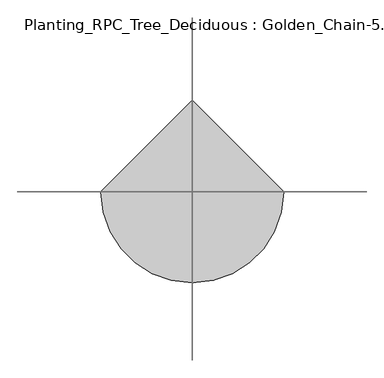
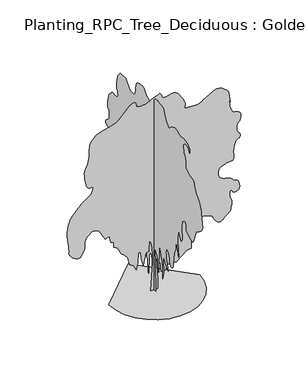
"""IFC4 building model written with IfcOpenShell, lengths in millimetres: geographic element geometry, Planting_RPC_Tree_Deciduous : Golden_Chain-5.5_Meters."""

from ifc_helpers import new_model, si_unit, origin, place, context, project, spatial, triangles, source, transform, mapped, element, save


def planting_rpc_tree_deciduous_golden_chain_5_5_meters_a00e3d8d(model_context):
    return source(origin(), model_context, "Body", "Tessellation", [
        triangles([(-0.0021492, 84.2526244, 0.0017055), (-0.0021492, -79.7118133, 0.0017055), (-0.0021492, -55.1171344, 770.634066), (-0.0021492, -30.52271, 1205.1392303), (-0.0021492, -128.9011709, 1090.3649134), (-0.0021492, -161.6941638, 983.7871164), (-0.0021492, -161.6941638, 778.8331295), (-0.0021492, -202.6851937, 614.866975), (-0.0021492, -227.2798771, 1410.0957607), (-0.0021492, -292.8648455, 1254.3285244), (-0.0021492, -391.2435608, 934.5977497), (-0.0021492, -407.6416878, 557.4810519), (-0.0021492, -448.631991, 754.2384825), (-0.0021492, -424.0373076, 1123.1586239), (-0.0021492, -399.4426243, 1229.73395), (-0.0021492, -563.406308, 1024.7799631), (-0.0021492, -645.3893852, 910.0031027), (-0.0021492, -571.6053715, 1164.1489271), (-0.0021492, -566.3701896, 1202.7023878), (-0.0021492, -561.3514189, 1240.6803749), (-0.0021492, -556.7629998, 1277.5125744), (-0.0021492, -552.8188002, 1312.6235126), (-0.0021492, -549.7352311, 1345.4427303), (-0.0021492, -547.7261968, 1375.3897396), (-0.0021492, -547.0106881, 1401.8966972), (-0.0021492, -548.2049103, 1425.0577835), (-0.0021492, -551.5507453, 1445.6369053), (-0.0021492, -556.6891671, 1464.0644142), (-0.0021492, -563.2636931, 1480.7706619), (-0.0021492, -570.9127902, 1496.1886162), (-0.0021492, -579.2773596, 1510.7457218), (-0.0021492, -588.000955, 1524.870005), (-0.0021492, -615.9185823, 1493.2475166), (-0.0021492, -642.6878059, 1461.6276443), (-0.0021492, -667.1627655, 1430.0051559), (-0.0021492, -688.1977461, 1398.3828129), (-0.0021492, -704.6417278, 1366.7627953), (-0.0021492, -715.3489231, 1335.1404522), (-0.0021492, -719.1734716, 1303.5179638), (-0.0021492, -720.8463346, 1273.0922047), (-0.0021492, -725.5315138, 1244.8155876), (-0.0021492, -732.7248247, 1218.3341372), (-0.0021492, -741.92717, 1193.2836313), (-0.0021492, -752.6342926, 1169.3103127), (-0.0021492, -764.3473131, 1146.0549734), (-0.0021492, -776.5592857, 1123.1586239), (-0.0021492, -799.2416948, 1123.4208899), (-0.0021492, -820.9921841, 1125.2619112), (-0.0021492, -840.8787609, 1130.2577545), (-0.0021492, -857.9695055, 1139.9845591), (-0.0021492, -871.3299545, 1156.0211529), (-0.0021492, -880.0306589, 1179.9486895), (-0.0021492, -883.1370827, 1213.3382938), (-0.0021492, -884.8100183, 1255.5711811), (-0.0021492, -889.4951975, 1304.2589069), (-0.0021492, -896.6885084, 1358.3243568), (-0.0021492, -905.890781, 1416.6931778), (-0.0021492, -916.5979763, 1478.2854939), (-0.0021492, -928.3109241, 1542.0320389), (-0.0021492, -940.5255129, 1606.8530823), (-0.0021492, -1006.1104631, 1762.6177025), (-0.0021492, -1030.7051828, 2041.3582466), (-0.0021492, -1137.2829798, 1615.049675), (-0.0021492, -1096.2901331, 2033.1591831), (-0.0021492, -1120.8847801, 2385.683741), (-0.0021492, -1260.2563602, 2139.7369801), (-0.0021492, -1270.7241806, 2153.8612633), (-0.0021492, -1280.7616493, 2168.4185143), (-0.0021492, -1289.9410309, 2183.833707), (-0.0021492, -1297.8295029, 2200.5425709), (-0.0021492, -1303.9940975, 2218.9700798), (-0.0021492, -1308.0095501, 2239.5492016), (-0.0021492, -1309.4456543, 2262.7104332), (-0.0021492, -1307.6275967, 2290.0779488), (-0.0021492, -1302.9424175, 2322.0339924), (-0.0021492, -1296.5385933, 2357.1449306), (-0.0021492, -1289.5590775, 2393.9769848), (-0.0021492, -1283.1526371, 2431.0969574), (-0.0021492, -1278.467458, 2467.0685989), (-0.0021492, -1276.6520164, 2500.4581306), (-0.0021492, -1277.8461296, 2532.7959824), (-0.0021492, -1281.1946171, 2566.4378242), (-0.0021492, -1286.3329662, 2601.1438454), (-0.0021492, -1292.9049488, 2636.6899315), (-0.0021492, -1300.5540459, 2672.8984772), (-0.0021492, -1308.9186516, 2709.5395546), (-0.0021492, -1317.642247, 2746.4099785), (-0.0021492, -1349.0965771, 2763.5973015), (-0.0021492, -1379.5477707, 2778.4931946), (-0.0021492, -1407.98993, 2788.7803574), (-0.0021492, -1433.4223892, 2792.1923584), (-0.0021492, -1454.8366344, 2786.4377678), (-0.0021492, -1471.2349068, 2769.1992851), (-0.0021492, -1481.6059307, 2738.2107697), (-0.0021492, -1484.4043064, 2701.9007767), (-0.0021492, -1481.8937038, 2669.6135033), (-0.0021492, -1478.8100258, 2640.331279), (-0.0021492, -1479.8871403, 2613.0602692), (-0.0021492, -1489.8533924, 2586.7825127), (-0.0021492, -1513.4448303, 2560.530336), (-0.0021492, -1555.3924152, 2533.2517685), (-0.0021492, -1606.8990097, 2505.0720932), (-0.0021492, -1655.2531803, 2478.4681938), (-0.0021492, -1699.3015091, 2456.025087), (-0.0021492, -1737.903368, 2440.3222664), (-0.0021492, -1769.9078098, 2433.9411152), (-0.0021492, -1794.1663582, 2439.4615631), (-0.0021492, -1809.5357689, 2459.4679001), (-0.0021492, -1957.1037964, 2820.1761154), (-0.0021492, -2096.4729057, 2918.565168), (-0.0021492, -2133.9034698, 2947.2108032), (-0.0021492, -2168.0339447, 2976.9770096), (-0.0021492, -2197.5760368, 3008.067263), (-0.0021492, -2221.2388367, 3040.5580124), (-0.0021492, -2237.731144, 3074.6530243), (-0.0021492, -2245.7621944, 3110.4540367), (-0.0021492, -2244.0409332, 3148.1136566), (-0.0021492, -2235.2459759, 3194.9401588), (-0.0021492, -2223.8691994, 3254.6760475), (-0.0021492, -2211.3439465, 3322.1530334), (-0.0021492, -2199.1064667, 3392.2016647), (-0.0021492, -2188.5902481, 3459.6786507), (-0.0021492, -2181.2289242, 3519.4145393), (-0.0021492, -2178.455983, 3566.2154617), (-0.0021492, -2170.3281361, 3608.6878693), (-0.0021492, -2147.5744377, 3658.060437), (-0.0021492, -2112.6316578, 3713.1367264), (-0.0021492, -2067.93395, 3772.8220367), (-0.0021492, -2015.9257874, 3835.9446373), (-0.0021492, -1959.038998, 3901.3845383), (-0.0021492, -1899.7154388, 3967.9447197), (-0.0021492, -1842.3295521, 4197.493499), (-0.0021492, -1629.1739582, 4246.6878799), (-0.0021492, -1457.0138271, 4328.6532257), (-0.0021492, -1458.3505188, 4335.1970123), (-0.0021492, -1461.6963902, 4352.7409996), (-0.0021492, -1466.0480141, 4378.3568779), (-0.0021492, -1470.3971672, 4408.9634399), (-0.0021492, -1473.7428932, 4441.6067963), (-0.0021492, -1475.0823463, 4473.206321), (-0.0021492, -1473.409338, 4500.8337044), (-0.0021492, -1467.7438408, 4526.8568253), (-0.0021492, -1458.2079403, 4555.4518822), (-0.0021492, -1445.4434578, 4586.2110512), (-0.0021492, -1430.0994816, 4618.7018005), (-0.0021492, -1412.8176876, 4652.465728), (-0.0021492, -1394.2476002, 4687.1208801), (-0.0021492, -1375.0306046, 4722.1832748), (-0.0021492, -1342.2369667, 4918.9358002), (-0.0021492, -1448.8147636, 5009.1256439), (-0.0021492, -1579.9871349, 4984.5283081), (-0.0021492, -1653.7686779, 4877.9400467), (-0.0021492, -1653.7686779, 4976.32939), (-0.0021492, -1538.9942883, 5082.8914902), (-0.0021492, -1350.4360302, 5107.488826), (-0.0021492, -1202.86793, 5074.692572), (-0.0021492, -1055.2998299, 5156.6834976), (-0.0021492, -948.7220329, 5164.8824158), (-0.0021492, -940.8820318, 5161.1390396), (-0.0021492, -920.1373678, 5151.1070938), (-0.0021492, -890.6410578, 5136.4911255), (-0.0021492, -856.5588358, 5118.9980072), (-0.0021492, -822.0437914, 5100.3340302), (-0.0021492, -791.2591152, 5082.280481), (-0.0021492, -768.3627657, 5066.4936539), (-0.0021492, -752.5401123, 5050.8591431), (-0.0021492, -739.1542288, 5033.7991379), (-0.0021492, -726.6289759, 5017.8844116), (-0.0021492, -713.388287, 5005.688063), (-0.0021492, -697.8532614, 4999.805864), (-0.0021492, -678.4454344, 5002.8359116), (-0.0021492, -653.5859053, 5017.2989822), (-0.0021492, -627.152853, 5039.5790176), (-0.0021492, -603.7294644, 5064.0234558), (-0.0021492, -582.8141713, 5090.2247635), (-0.0021492, -563.9079125, 5117.8777267), (-0.0021492, -546.5090836, 5146.6253906), (-0.0021492, -530.1109202, 5176.0608032), (-0.0021492, -514.2169413, 5205.8775879), (-0.0021492, -415.8382442, 5410.8290314), (-0.0021492, -169.8924643, 5451.8247849), (-0.0021492, -163.845268, 5451.6718872), (-0.0021492, -147.6161895, 5450.6789246), (-0.0021492, -124.0728773, 5447.9540909), (-0.0021492, -96.0842423, 5442.6323227), (-0.0021492, -66.5181782, 5433.8985535), (-0.0021492, -38.242574, 5420.8359787), (-0.0021492, -14.1260636, 5402.6301132), (-0.0021492, 3.3458591, 5384.2457703), (-0.0021492, 15.2248417, 5370.0373352), (-0.0021492, 23.9488607, 5358.0956223), (-0.0021492, 31.9557666, 5346.6114395), (-0.0021492, 41.6836385, 5333.6761826), (-0.0021492, 55.5706315, 5317.4312439), (-0.0021492, 76.0543103, 5296.0418518), (-0.0021492, 97.1353591, 5271.2921997), (-0.0021492, 113.1971422, 5247.5349289), (-0.0021492, 127.251426, 5226.7827072), (-0.0021492, 142.3092006, 5211.0464584), (-0.0021492, 161.3827366, 5202.3638489), (-0.0021492, 187.4830512, 5202.6946426), (-0.0021492, 223.6221243, 5214.0770874), (-0.0021492, 264.3514152, 5233.7851868), (-0.0021492, 302.4974698, 5257.3895599), (-0.0021492, 338.4919115, 5284.2018768), (-0.0021492, 372.7676173, 5313.5861298), (-0.0021492, 405.7523409, 5344.9307281), (-0.0021492, 437.8764338, 5377.549086), (-0.0021492, 469.5676317, 5410.8290314), (-0.0021492, 492.4664884, 5419.4866425), (-0.0021492, 515.7217913, 5427.329187), (-0.0021492, 539.6951826, 5433.618338), (-0.0021492, 564.7456521, 5437.5396103), (-0.0021492, 591.2271389, 5438.3035172), (-0.0021492, 619.503756, 5435.1205719), (-0.0021492, 649.9294424, 5427.227449), (-0.0021492, 681.4067362, 5417.9076691), (-0.0021492, 712.0260155, 5409.8616486), (-0.0021492, 740.9213448, 5401.4080948), (-0.0021492, 767.2373257, 5390.7895569), (-0.0021492, 790.1107115, 5376.3014877), (-0.0021492, 808.683415, 5356.2364334), (-0.0021492, 822.0921896, 5328.8381058), (-0.0021492, 831.6764883, 5297.4679276), (-0.0021492, 839.5394531, 5266.5052826), (-0.0021492, 845.9687845, 5235.9240097), (-0.0021492, 851.252401, 5205.5973724), (-0.0021492, 855.6727707, 5175.5259521), (-0.0021492, 859.5227537, 5145.5556885), (-0.0021492, 863.0824928, 5115.6877441), (-0.0021492, 868.5086151, 5085.9982773), (-0.0021492, 874.8667299, 5057.4029297), (-0.0021492, 883.0887571, 5030.9469864), (-0.0021492, 894.1065439, 5007.6995682), (-0.0021492, 908.8546989, 4988.7803741), (-0.0021492, 928.2625986, 4975.2085281), (-0.0021492, 953.2646336, 4968.1298904), (-0.0021492, 983.5707052, 4964.7946289), (-0.0021492, 1017.0341423, 4962.6302261), (-0.0021492, 1051.7859455, 4962.7319641), (-0.0021492, 1085.9648912, 4966.2968628), (-0.0021492, 1117.7070671, 4974.4446213), (-0.0021492, 1145.1459446, 4988.3478424), (-0.0021492, 1166.417684, 5009.1256439), (-0.0021492, 1187.9516893, 5037.6186722), (-0.0021492, 1215.2250973, 5071.5857849), (-0.0021492, 1244.9327316, 5107.4126678), (-0.0021492, 1273.7822788, 5141.5326782), (-0.0021492, 1298.4736496, 5170.3315018), (-0.0021492, 1315.7070454, 5190.2436584), (-0.0021492, 1322.1822315, 5197.6786697), (-0.0021492, 1576.3282013, 5181.2802521), (-0.0021492, 1674.7067894, 5058.2941544), (-0.0021492, 1679.9878624, 5049.3057495), (-0.0021492, 1685.3427681, 5039.1209061), (-0.0021492, 1690.8402523, 5026.4658646), (-0.0021492, 1696.5540024, 5010.1691849), (-0.0021492, 1702.550584, 4988.9844315), (-0.0021492, 1708.9087715, 4961.7134216), (-0.0021492, 1715.6971653, 4927.1347183), (-0.0021492, 1722.2461842, 4888.9655365), (-0.0021492, 1727.9346451, 4851.6622902), (-0.0021492, 1732.9075974, 4815.0467926), (-0.0021492, 1737.3050034, 4779.0420135), (-0.0021492, 1741.2720577, 4743.4447678), (-0.0021492, 1744.9541004, 4708.1530266), (-0.0021492, 1748.4909485, 4672.9888939), (-0.0021492, 1731.0895397, 4648.3406891), (-0.0021492, 1714.6938835, 4623.4122688), (-0.0021492, 1700.3047909, 4597.923999), (-0.0021492, 1688.927869, 4571.5442139), (-0.0021492, 1681.5665451, 4544.0444389), (-0.0021492, 1679.2239555, 4515.0930084), (-0.0021492, 1682.9058529, 4484.4355774), (-0.0021492, 1691.9172215, 4457.546521), (-0.0021492, 1704.7989933, 4438.9587021), (-0.0021492, 1721.4110607, 4426.9911186), (-0.0021492, 1741.6082291, 4419.8869011), (-0.0021492, 1765.2454491, 4415.940049), (-0.0021492, 1792.1827583, 4413.4448524), (-0.0021492, 1822.2749622, 4410.6438606), (-0.0021492, 1851.5776794, 4410.5165428), (-0.0021492, 1877.0101387, 4414.7180305), (-0.0021492, 1899.7154388, 4419.4540787), (-0.0021492, 1920.8445271, 4421.0583412), (-0.0021492, 1941.543409, 4415.787442), (-0.0021492, 1962.9577995, 4399.8985863), (-0.0021492, 1986.2386459, 4369.6483978), (-0.0021492, 2009.8529022, 4339.0165466), (-0.0021492, 2031.6034641, 4320.2758301), (-0.0021492, 2051.6326195, 4307.2641243), (-0.0021492, 2070.0855629, 4293.8451759), (-0.0021492, 2087.1025475, 4273.8059921), (-0.0021492, 2102.8309479, 4241.0097382), (-0.0021492, 2117.4110172, 4189.2942902), (-0.0021492, 2130.4608021, 4132.1300468), (-0.0021492, 2141.5041687, 4085.4564423), (-0.0021492, 2150.5383556, 4046.6762512), (-0.0021492, 2157.5661243, 4013.1925392), (-0.0021492, 2162.5848587, 3982.4330795), (-0.0021492, 2165.5945587, 3951.8012283), (-0.0021492, 2166.6004566, 3918.7503387), (-0.0021492, 2163.9700939, 3888.1437767), (-0.0021492, 2156.60877, 3865.7364235), (-0.0021492, 2145.3032101, 3850.1274925), (-0.0021492, 2130.8427555, 3839.9679382), (-0.0021492, 2114.016893, 3833.907843), (-0.0021492, 2095.6122025, 3830.546711), (-0.0021492, 2076.4181705, 3828.560495), (-0.0021492, 2076.4181705, 3615.4101334), (-0.0021492, 2076.5863289, 3611.7687859), (-0.0021492, 2077.7576237, 3607.2365044), (-0.0021492, 2080.9353367, 3600.9979317), (-0.0021492, 2087.1279819, 3592.1877136), (-0.0021492, 2097.3334637, 3579.9146255), (-0.0021492, 2112.5578251, 3563.3636009), (-0.0021492, 2133.8066734, 3541.6437057), (-0.0021492, 2158.6890209, 3518.82911), (-0.0021492, 2183.2837406, 3498.7640556), (-0.0021492, 2206.2997776, 3480.0997879), (-0.0021492, 2226.4485477, 3461.613707), (-0.0021492, 2242.4392868, 3441.9561859), (-0.0021492, 2252.9809399, 3419.8799171), (-0.0021492, 2256.7799812, 3394.0605629), (-0.0021492, 2250.3277588, 3369.7687317), (-0.0021492, 2232.2566235, 3352.3776421), (-0.0021492, 2204.5071545, 3340.7155632), (-0.0021492, 2169.0142628, 3333.6369255), (-0.0021492, 2127.7108246, 3329.995578), (-0.0021492, 2082.5369831, 3328.6715309), (-0.0021492, 2035.42794, 3328.4677643), (-0.0021492, 2021.5658501, 3329.995578), (-0.0021492, 2008.8497658, 3330.1737648), (-0.0021492, 1998.4277275, 3327.6276993), (-0.0021492, 1991.4508278, 3320.981884), (-0.0021492, 1989.05984, 3308.8869827), (-0.0021492, 1992.4057114, 3289.9677887), (-0.0021492, 2002.6367729, 3262.9008362), (-0.0021492, 2020.3945553, 3234.9679482), (-0.0021492, 2044.3195484, 3213.2224731), (-0.0021492, 2072.5479126, 3195.7802238), (-0.0021492, 2103.2129013, 3180.7573036), (-0.0021492, 2134.4508202, 3166.3198128), (-0.0021492, 2164.4004456, 3150.6091438), (-0.0021492, 2191.195031, 3131.7155296), (-0.0021492, 2214.6668541, 3115.4703003), (-0.0021492, 2235.4115181, 3106.0996513), (-0.0021492, 2252.7161304, 3099.4538361), (-0.0021492, 2265.8627117, 3091.3822357), (-0.0021492, 2274.1329918, 3077.7086517), (-0.0021492, 2276.8092819, 3054.282756), (-0.0021492, 2273.1756374, 3016.9539299), (-0.0021492, 2263.7594971, 2975.5765137), (-0.0021492, 2250.0399857, 2941.9401947), (-0.0021492, 2232.7353733, 2914.7709229), (-0.0021492, 2212.5636395, 2892.7455231), (-0.0021492, 2190.2376766, 2874.6161064), (-0.0021492, 2166.4806965, 2859.0580444), (-0.0021492, 2142.0057369, 2844.7734512), (-0.0021492, 2133.3763218, 2827.178595), (-0.0021492, 2125.6814426, 2809.2779434), (-0.0021492, 2119.8477871, 2790.7918625), (-0.0021492, 2116.8126526, 2771.4654259), (-0.0021492, 2117.5051975, 2750.9678398), (-0.0021492, 2122.8601032, 2729.044178), (-0.0021492, 2133.8066734, 2705.4145157), (-0.0021492, 2153.6932503, 2682.9815826), (-0.0021492, 2182.4714355, 2663.4008011), (-0.0021492, 2215.9807274, 2644.532476), (-0.0021492, 2250.0629494, 2624.2386566), (-0.0021492, 2280.5623959, 2600.3543587), (-0.0021492, 2303.3160942, 2570.74105), (-0.0021492, 2314.1684841, 2533.2517685), (-0.0021492, 2316.6306885, 2491.7827881), (-0.0021492, 2316.7962307, 2450.4565315), (-0.0021492, 2314.3824245, 2407.4087231), (-0.0021492, 2309.1013515, 2360.7784298), (-0.0021492, 2300.6629131, 2308.6964344), (-0.0021492, 2288.7844231, 2249.3015133), (-0.0021492, 2273.1756374, 2180.7272106), (-0.0021492, 2256.9481396, 2122.3126076), (-0.0021492, 2242.7270599, 2087.8459614), (-0.0021492, 2229.5092621, 2067.1472248), (-0.0021492, 2216.2913189, 2050.0334438), (-0.0021492, 2202.0703846, 2026.3248619), (-0.0021492, 2185.8402706, 1985.8337288), (-0.0021492, 2166.6004566, 1918.3849388), (-0.0021492, 2149.5810013, 1842.5205288), (-0.0021492, 2138.873806, 1783.2936207), (-0.0021492, 2131.751857, 1740.2713921), (-0.0021492, 2125.4904659, 1713.0234913), (-0.0021492, 2117.362619, 1701.1195667), (-0.0021492, 2104.6465347, 1704.1318829), (-0.0021492, 2084.617234, 1721.6274719), (-0.0021492, 2060.5012642, 1758.077718), (-0.0021492, 2037.2459976, 1813.4570412), (-0.0021492, 2014.7062397, 1880.5978558), (-0.0021492, 1992.7392666, 1952.324437), (-0.0021492, 1971.2052612, 2021.4716698), (-0.0021492, 1949.9564129, 2080.8665909), (-0.0021492, 1928.8527592, 2123.3388531), (-0.0021492, 1903.2293232, 2154.4825916), (-0.0021492, 1869.4322582, 2184.768243), (-0.0021492, 1828.8239811, 2214.3332989), (-0.0021492, 1782.766618, 2243.3254246), (-0.0021492, 1732.6198242, 2271.8871986), (-0.0021492, 1679.7511036, 2300.1638157), (-0.0021492, 1625.5174953, 2328.2953835), (-0.0021492, 1580.1042789, 2357.6694626), (-0.0021492, 1536.2697453, 2384.1050583), (-0.0021492, 1495.5901062, 2404.6613617), (-0.0021492, 1459.6415737, 2416.3971279), (-0.0021492, 1430.0026852, 2416.3716934), (-0.0021492, 1408.2522686, 2401.6490456), (-0.0021492, 1395.9662453, 2369.285614), (-0.0021492, 1387.7443634, 2327.3633183), (-0.0021492, 1377.3731941, 2285.8715195), (-0.0021492, 1365.2070763, 2244.7360943), (-0.0021492, 1351.607325, 2203.8884422), (-0.0021492, 1336.9304592, 2163.2545853), (-0.0021492, 1321.5380848, 2122.7659229), (-0.0021492, 1305.7867207, 2082.3484772), (-0.0021492, 1125.4248373, 1926.5840023), (-0.0021492, 1107.9776464, 1907.1276318), (-0.0021492, 1091.2458916, 1886.8820652), (-0.0021492, 1075.9503136, 1865.0602867), (-0.0021492, 1062.803805, 1840.8731003), (-0.0021492, 1052.5269613, 1813.5284031), (-0.0021492, 1045.8352913, 1782.242086), (-0.0021492, 1043.4443035, 1746.2221916), (-0.0021492, 1042.7262514, 1711.1596516), (-0.0021492, 1040.7197605, 1682.5468632), (-0.0021492, 1037.6362278, 1659.3170311), (-0.0021492, 1033.6919918, 1640.3853378), (-0.0021492, 1029.1035364, 1624.6823719), (-0.0021492, 1024.0848021, 1611.1308735), (-0.0021492, 1018.8495838, 1598.6540188), (-0.0021492, 871.2815563, 1500.2752853), (-0.0021492, 854.8859728, 1328.1125381), (-0.0021492, 731.9125923, 1270.7241806), (-0.0021492, 699.1188091, 1057.5711302), (-0.0021492, 567.9463288, 1024.7799631), (-0.0021492, 579.9928682, 1019.3537682), (-0.0021492, 590.5345213, 1012.9956533), (-0.0021492, 598.0639309, 1004.7736988), (-0.0021492, 601.0736672, 993.7558393), (-0.0021492, 598.0639309, 979.0076843), (-0.0021492, 587.5222778, 959.5998573), (-0.0021492, 567.9463288, 934.5977497), (-0.0021492, 544.3090725, 908.8801334), (-0.0021492, 522.3905339, 887.4632721), (-0.0021492, 501.9081359, 869.6341278), (-0.0021492, 482.5715618, 854.6720324), (-0.0021492, 464.0956547, 841.8616224), (-0.0021492, 446.1926414, 830.4822298), (-0.0021492, 428.5773648, 819.8234327), (-0.0021492, 416.3169213, 852.4975285), (-0.0021492, 404.2704183, 880.9396877), (-0.0021492, 392.6541942, 900.9204449), (-0.0021492, 381.6821895, 908.2104795), (-0.0021492, 371.5733952, 898.5778553), (-0.0021492, 362.5365921, 867.7931065), (-0.0021492, 354.7933147, 811.6243692), (-0.0021492, 347.289376, 757.5588467), (-0.0021492, 338.9222631, 728.4470335), (-0.0021492, 329.8396053, 713.1030573), (-0.0021492, 320.1840537, 700.3410456), (-0.0021492, 310.0981868, 678.9725098), (-0.0021492, 299.7245649, 637.8141935), (-0.0021492, 289.2083645, 565.6776083), (-0.0021492, 280.100254, 485.3215756), (-0.0021492, 273.5766333, 424.7553597), (-0.0021492, 269.2021002, 380.6815238), (-0.0021492, 266.5488646, 349.8000149), (-0.0021492, 265.1865931, 328.8160123), (-0.0021492, 264.6849704, 314.4268833), (-0.0021492, 264.6136811, 303.3352093), (-0.0021492, 240.0187434, 811.6243692), (-0.0021492, 227.6618305, 844.6574547), (-0.0021492, 214.9461277, 875.6102892), (-0.0021492, 201.5133903, 902.4024038), (-0.0021492, 187.005355, 922.9586346), (-0.0021492, 171.062996, 935.1961143), (-0.0021492, 153.3280502, 937.0371357), (-0.0021492, 133.441982, 926.4012297), (-0.0021492, 115.7070271, 904.2917507), (-0.0021492, 103.9950785, 874.0086428), (-0.0021492, 97.3026454, 836.9141773), (-0.0021492, 94.6257285, 794.3681551), (-0.0021492, 94.9603102, 747.7377892), (-0.0021492, 97.3026454, 698.3804094), (-0.0021492, 100.6487348, 647.6606855), (-0.0021492, 84.2526244, 237.7500047), (88.443575, 0.0002505, 0.0), (-86.3932913, 0.0002505, 0.0), (-44.7656769, 0.0002025, 807.5808661), (-36.4400495, 0.0001919, 1032.3704882), (-69.7422955, 0.0001759, 1307.1158546), (-128.0216733, 0.0001652, 1448.6492214), (-144.6726737, 0.0001865, 1140.603344), (-227.9279117, 0.0001865, 1115.6267435), (-294.532658, 0.0002025, 799.2544847), (-352.8122947, 0.0001919, 999.0699772), (-361.138676, 0.0001812, 1182.2301636), (-427.7421687, 0.0001812, 1182.2301636), (-444.3923879, 0.0001972, 915.8137218), (-486.0217873, 0.0002079, 732.650992), (-552.62528, 0.0002025, 874.1843588), (-660.8581358, 0.0001972, 940.7903223), (-702.4850281, 0.0001812, 1157.2535631), (-785.7412834, 0.0001759, 1257.1626537), (-877.3239201, 0.0001759, 1332.0925278), (-977.2303946, 0.0001599, 1523.5790955), (-1085.4632504, 0.0001599, 1581.8586777), (-1085.4632504, 0.0001492, 1723.3945152), (-1160.3931244, 0.0001492, 1748.3711884), (-1202.0200167, 0.0001386, 1939.857756), (-1318.5792538, 0.0001386, 1889.9045551), (-1468.4390018, 0.0001226, 2172.9737595), (-1502.3251602, 0.0001226, 2194.044421), (-1536.1348698, 0.0001226, 2213.0729107), (-1569.8020008, 0.0001173, 2228.0247597), (-1603.2501045, 0.0001173, 2236.8604122), (-1636.4054935, 0.0001173, 2237.5401672), (-1669.1992767, 0.0001173, 2228.0247597), (-1701.5550053, 0.0001226, 2206.2768139), (-1733.4728245, 0.0001226, 2179.0187393), (-1764.2270519, 0.0001226, 2153.3621658), (-1792.6513344, 0.0001279, 2127.8509323), (-1817.5796093, 0.0001279, 2101.0307671), (-1837.8479942, 0.0001279, 2071.4427475), (-1852.2881012, 0.0001332, 2037.6304218), (-1859.7411346, 0.0001332, 1998.1374836), (-1862.0709343, 0.0001386, 1954.9318359), (-1863.0894768, 0.0001386, 1911.4360897), (-1864.5459286, 0.0001439, 1868.3756367), (-1868.1871307, 0.0001439, 1826.4813915), (-1875.7599243, 0.0001439, 1786.4790367), (-1889.0133305, 0.0001492, 1749.0994869), (-1909.6943356, 0.0001492, 1715.0681339), (-1930.6657299, 0.0001546, 1683.7079842), (-1945.9586918, 0.0001546, 1654.8228287), (-1959.0645779, 0.0001546, 1629.87159), (-1973.4841919, 0.0001546, 1610.3059238), (-1992.7087452, 0.0001599, 1597.5872234), (-2020.2342453, 0.0001599, 1593.1693245), (-2059.5540836, 0.0001599, 1598.5089695), (-2106.0851097, 0.0001546, 1614.4818317), (-2151.452544, 0.0001546, 1639.629134), (-2193.466404, 0.0001546, 1671.9110298), (-2229.9497875, 0.0001492, 1709.2905796), (-2258.7127121, 0.0001492, 1749.7309891), (-2277.5730434, 0.0001439, 1791.1871796), (-2284.3437057, 0.0001439, 1831.6274437), (-2284.0050636, 0.0001439, 1867.2348633), (-2283.6664215, 0.0001386, 1899.3462753), (-2284.3437057, 0.0001386, 1933.6447632), (-2287.0631618, 0.0001332, 1975.8064339), (-2292.8407162, 0.0001332, 2031.5117546), (-2302.6949112, 0.0001279, 2106.4440994), (-2317.6467602, 0.0001226, 2206.2768139), (-2328.3767738, 0.0001119, 2318.4666229), (-2327.0171185, 0.0001066, 2424.8304794), (-2316.773267, 0.0001013, 2522.6006744), (-2300.8512737, 9.59e-05, 2609.0116791), (-2282.4518154, 9.06e-05, 2681.301162), (-2264.7805103, 9.06e-05, 2736.6829559), (-2251.0432674, 8.53e-05, 2772.4075195), (-2228.7606159, 8.53e-05, 2807.0373825), (-2187.9817097, 7.99e-05, 2856.639006), (-2135.6985638, 7.99e-05, 2914.8473717), (-2078.9008678, 7.46e-05, 2975.2457199), (-2024.5781662, 7.46e-05, 3031.4170006), (-1979.7200031, 6.93e-05, 3076.9447449), (-1951.3211552, 6.93e-05, 3105.4377731), (-1924.2821079, 6.4e-05, 3127.0812195), (-1882.8233013, 6.4e-05, 3155.294323), (-1832.9184986, 6.4e-05, 3188.4469505), (-1780.5385563, 5.86e-05, 3224.9610008), (-1731.6521507, 5.86e-05, 3263.2063408), (-1692.2330452, 5.33e-05, 3301.6042877), (-1668.2519508, 5.33e-05, 3338.5511604), (-1656.1647526, 5.33e-05, 3371.3221252), (-1648.0090004, 4.8e-05, 3398.84748), (-1643.1302284, 4.8e-05, 3421.9934509), (-1640.8716454, 4.8e-05, 3441.6762611), (-1640.5814014, 4.8e-05, 3458.7109772), (-1641.5999439, 4.8e-05, 3473.9888237), (-1643.275423, 4.26e-05, 3488.4263145), (-1673.4947994, 4.26e-05, 3483.4864998), (-1703.0598553, 4.26e-05, 3481.1183304), (-1731.3135086, 4.26e-05, 3483.8172935), (-1757.6015842, 4.26e-05, 3494.1809052), (-1781.2668549, 4.26e-05, 3514.75494), (-1801.657616, 4.26e-05, 3548.0604652), (-1818.114315, 3.73e-05, 3596.643837), (-1832.6281094, 3.2e-05, 3658.2386238), (-1846.5615612, 3.2e-05, 3726.3521988), (-1858.3075012, 2.66e-05, 3797.4193726), (-1866.2698059, 2.13e-05, 3867.7226395), (-1868.8440674, 1.6e-05, 3933.671521), (-1864.4263138, 1.6e-05, 3991.625251), (-1851.4147533, 1.07e-05, 4037.891613), (-1831.8515579, 1.07e-05, 4080.6183655), (-1810.1036121, 5.3e-06, 4129.8891953), (-1788.0628063, 5.3e-06, 4185.1439621), (-1767.626263, 0.0, 4245.7710754), (-1750.6832565, -5.3e-06, 4311.2109764), (-1739.1281479, -1.07e-05, 4380.8776543), (-1734.8580597, -1.07e-05, 4454.1856796), (-1735.4895618, -1.6e-05, 4523.8776466), (-1735.828204, -2.13e-05, 4584.5303398), (-1733.5466572, -2.13e-05, 4638.3337418), (-1726.3126511, -2.66e-05, 4687.5028336), (-1711.7987114, -3.2e-05, 4734.1764381), (-1687.670097, -3.2e-05, 4780.5442474), (-1651.6018044, -3.73e-05, 4828.8221146), (-1604.6581581, -3.73e-05, 4875.2410835), (-1551.3057461, -4.26e-05, 4914.6575729), (-1494.3144573, -4.26e-05, 4947.2247711), (-1436.4473499, -4.26e-05, 4973.1208649), (-1380.4746037, -4.26e-05, 4992.421431), (-1329.1617474, -4.8e-05, 5005.3566879), (-1285.2761993, -4.8e-05, 5012.0027939), (-1238.8191513, -4.8e-05, 5019.8197586), (-1181.7285954, -4.8e-05, 5034.7665207), (-1119.6855074, -4.8e-05, 5054.8059952), (-1058.3732615, -4.8e-05, 5077.9260956), (-1003.4674559, -5.33e-05, 5102.03974), (-960.6514647, -5.33e-05, 5125.1604218), (-935.6010315, -5.33e-05, 5145.1993149), (-669.1845171, -6.93e-05, 5428.27099), (-646.0030832, -6.93e-05, 5444.1601364), (-622.8954094, -7.46e-05, 5458.928421), (-599.9329302, -7.46e-05, 5471.5328842), (-577.1894056, -7.46e-05, 5480.8520828), (-554.7387048, -7.46e-05, 5485.7918976), (-532.6495734, -7.46e-05, 5485.2826263), (-510.9984241, -7.46e-05, 5478.2295685), (-495.8275841, -7.46e-05, 5462.4933197), (-489.5407948, -6.93e-05, 5439.0418442), (-486.7500495, -6.93e-05, 5411.3894623), (-482.0648704, -6.93e-05, 5382.9725922), (-470.0972506, -6.93e-05, 5357.3567139), (-445.4618357, -6.4e-05, 5337.9794083), (-402.7655319, -6.4e-05, 5328.3544144), (-352.155358, -6.4e-05, 5326.9794983), (-306.7905398, -6.4e-05, 5329.5258545), (-265.7951679, -6.4e-05, 5335.3568939), (-228.2925333, -6.4e-05, 5343.8104477), (-193.4123586, -6.4e-05, 5354.2249283), (-160.2802058, -6.93e-05, 5365.9381668), (-128.0216733, -6.93e-05, 5378.3129929), (-76.4902348, -6.93e-05, 5408.3594147), (-26.1968067, -6.93e-05, 5436.750705), (21.6206802, -7.46e-05, 5461.7805725), (65.7244948, -7.46e-05, 5481.7688873), (104.8766017, -7.46e-05, 5495.0605179), (137.8389248, -7.46e-05, 5500.0003326), (163.3739486, -7.46e-05, 5494.8826218), (179.7578323, -7.46e-05, 5482.2525787), (188.4231464, -7.46e-05, 5466.2872742), (192.8648993, -7.46e-05, 5447.6994553), (196.5786806, -6.93e-05, 5427.2018692), (203.0594986, -6.93e-05, 5405.5584229), (215.802707, -6.93e-05, 5383.4562836), (238.3035683, -6.93e-05, 5361.6599396), (275.7078986, -6.4e-05, 5352.0099472), (327.5301169, -6.93e-05, 5359.8269119), (388.8194718, -6.93e-05, 5376.0974304), (454.6234131, -6.93e-05, 5391.7575211), (519.9894087, -6.93e-05, 5397.8431961), (579.9673974, -6.93e-05, 5385.2643127), (629.6048836, -6.4e-05, 5345.0074677), (669.510442, -6.4e-05, 5289.625383), (704.1732244, -5.86e-05, 5237.2989258), (734.4639627, -5.86e-05, 5187.5188248), (761.2611643, -5.33e-05, 5139.7758087), (785.4382496, -5.33e-05, 5093.5606064), (807.8660231, -4.8e-05, 5048.3639465), (829.4204487, -4.8e-05, 5003.6765579), (821.0940674, -3.73e-05, 4853.8014038), (1104.1632717, -3.73e-05, 4837.1486412), (1130.9121477, -3.73e-05, 4839.0836975), (1157.5871183, -3.73e-05, 4841.7826607), (1184.116967, -3.73e-05, 4846.1114662), (1210.4304045, -3.73e-05, 4852.8337303), (1236.4509819, -3.73e-05, 4862.7642288), (1262.1075554, -3.73e-05, 4876.6924484), (1287.3260742, -3.73e-05, 4895.433165), (1317.642247, -4.26e-05, 4918.5538467), (1357.5732399, -4.26e-05, 4944.7039948), (1405.5098488, -4.26e-05, 4973.4260788), (1459.8579849, -4.8e-05, 5004.1858292), (1519.0110603, -4.8e-05, 5036.4728119), (1581.3672832, -4.8e-05, 5069.7527573), (1645.3251526, -5.33e-05, 5103.5675537), (1684.4540142, -5.33e-05, 5099.8497574), (1722.8522518, -5.33e-05, 5095.2668976), (1759.7965084, -5.33e-05, 5088.9515854), (1794.5558693, -4.8e-05, 5079.9887604), (1826.3998558, -4.8e-05, 5067.5371948), (1854.6052563, -4.8e-05, 5050.7062454), (1878.441156, -4.8e-05, 5028.6552658), (1900.2145363, -4.8e-05, 5007.1902969), (1922.1329659, -4.26e-05, 4990.5372437), (1943.3232422, -4.26e-05, 4975.3358459), (1962.9120174, -4.26e-05, 4958.2502609), (1980.023037, -4.26e-05, 4935.9196472), (1993.7858597, -3.73e-05, 4905.0075806), (2003.3268471, -3.73e-05, 4862.1276398), (2036.6272854, -2.13e-05, 4620.6877258), (2031.3360386, -2.66e-05, 4643.2226875), (2026.4090137, -2.66e-05, 4661.7340576), (2022.2101421, -2.66e-05, 4672.2502762), (2019.1036457, -2.66e-05, 4670.7480423), (2017.4511303, -2.66e-05, 4653.2296349), (2017.6217594, -2.13e-05, 4615.6717529), (2019.9769936, -2.13e-05, 4554.0766754), (2029.0544918, -1.6e-05, 4483.8245682), (2046.7257969, -1.07e-05, 4423.1715843), (2069.3470905, -5.3e-06, 4372.5514183), (2093.2797867, -5.3e-06, 4332.4216003), (2114.8825378, -5.3e-06, 4303.241114), (2130.5142872, -5.3e-06, 4285.3916222), (2136.5336872, 0.0, 4279.3568161), (2147.5540901, 0.0, 4280.1463028), (2175.7594906, 0.0, 4279.6370316), (2213.8673389, 0.0, 4273.4493279), (2254.597847, 0.0, 4257.2040985), (2290.6661396, 0.0, 4226.5466675), (2314.7948994, 5.3e-06, 4177.0976509), (2319.6964897, 1.07e-05, 4104.5026634), (2308.0217663, 1.07e-05, 4035.0650414), (2289.5025478, 1.6e-05, 3991.3961952), (2267.4871765, 1.6e-05, 3963.6159142), (2245.3242851, 1.6e-05, 3941.794281), (2226.3696281, 2.13e-05, 3916.0257957), (2213.9641354, 2.13e-05, 3876.4308289), (2211.4661774, 2.66e-05, 3813.1044617), (2219.5964951, 2.66e-05, 3747.2826073), (2234.7189732, 3.2e-05, 3702.4170319), (2253.6252319, 3.2e-05, 3671.9886566), (2273.1170654, 3.73e-05, 3649.4284058), (2289.9862392, 3.73e-05, 3628.1416237), (2301.0320766, 3.73e-05, 3601.6601006), (2303.0461979, 4.26e-05, 3563.3383118), (2294.2843781, 4.26e-05, 3529.0395332), (2276.7837021, 4.26e-05, 3512.2341637), (2253.0191643, 4.26e-05, 3502.8382256), (2225.4708458, 4.26e-05, 3490.8197731), (2196.6085087, 4.8e-05, 3466.1206993), (2168.9149956, 4.8e-05, 3418.7340569), (2144.8600685, 5.33e-05, 3338.5511604), (2129.882785, 5.86e-05, 3243.8799042), (2124.958231, 6.4e-05, 3160.2850067), (2125.8545425, 6.93e-05, 3088.6321129), (2128.3549713, 7.46e-05, 3029.812738), (2128.2327404, 7.46e-05, 2984.6669472), (2121.2661598, 7.46e-05, 2954.085965), (2103.2332489, 7.99e-05, 2938.9354362), (2080.3674934, 7.99e-05, 2933.5627991), (2059.9793484, 7.99e-05, 2930.6853584), (2039.4433926, 7.99e-05, 2928.6482735), (2016.1423439, 7.99e-05, 2925.9237305), (1987.4506359, 7.99e-05, 2920.8565979), (1950.7508411, 7.99e-05, 2911.8429039), (1903.4176838, 7.99e-05, 2897.3033844), (1853.5128811, 7.99e-05, 2880.1413506), (1811.035532, 7.99e-05, 2862.9793167), (1776.2786419, 8.53e-05, 2843.7801979), (1749.5298386, 8.53e-05, 2820.5071999), (1731.0818367, 8.53e-05, 2791.0973671), (1721.2276417, 9.06e-05, 2753.565065), (1720.2574974, 9.06e-05, 2705.822049), (1723.6314194, 9.59e-05, 2658.5118553), (1727.8785439, 9.59e-05, 2621.9725159), (1734.8910519, 9.59e-05, 2593.7341232), (1746.5683914, 0.0001013, 2571.3520592), (1764.7947498, 0.0001013, 2552.2802582), (1791.4723366, 0.0001013, 2534.1049141), (1828.4878098, 0.0001013, 2514.3226913), (1873.0047146, 0.0001013, 2496.0453186), (1919.5613205, 0.0001066, 2482.2824959), (1966.1151649, 0.0001066, 2470.414325), (2010.6320698, 0.0001066, 2457.8153847), (2051.0698631, 0.0001066, 2441.8678116), (2085.3913147, 0.0001066, 2419.9518528), (2111.5571594, 0.0001119, 2389.4394711), (2135.6603394, 0.0001119, 2361.7918854), (2163.6951107, 0.0001119, 2345.6508648), (2193.4790485, 0.0001119, 2334.1695889), (2222.8252224, 0.0001119, 2320.5061787), (2249.5485912, 0.0001173, 2297.8085815), (2271.4670208, 0.0001173, 2259.2397148), (2286.3960514, 0.0001226, 2197.9504326), (2290.302063, 0.0001279, 2132.9740208), (2281.9781525, 0.0001279, 2085.908289), (2263.4564632, 0.0001279, 2053.7714424), (2236.7814926, 0.0001332, 2033.5767448), (2203.9877094, 0.0001332, 2022.3374599), (2167.1172855, 0.0001332, 2017.0716476), (2128.209922, 0.0001332, 2014.7876301), (2106.9228493, 0.0001332, 2046.2217579), (2086.3640751, 0.0001279, 2073.5764835), (2067.2591366, 0.0001279, 2092.7782185), (2050.3415646, 0.0001279, 2099.7423283), (2036.3368961, 0.0001279, 2090.3974045), (2025.9709591, 0.0001279, 2060.6643356), (2019.9769936, 0.0001332, 2006.4638649), (2022.332373, 0.0001386, 1947.8938934), (2033.7142365, 0.0001386, 1903.8862598), (2049.9036552, 0.0001439, 1868.6174824), (2066.6760326, 0.0001439, 1836.2617538), (2079.809824, 0.0001439, 1800.9929764), (2085.0756363, 0.0001492, 1756.9878136), (2078.254105, 0.0001492, 1698.4179874), (2066.0701103, 0.0001546, 1638.7047718), (2056.2159153, 0.0001599, 1592.8306824), (2045.923811, 0.0001599, 1557.2946247), (2032.4284138, 0.0001599, 1528.6053875), (2012.9620148, 0.0001652, 1503.2646378), (1984.7566143, 0.0001652, 1477.7762226), (1945.0471195, 0.0001652, 1448.6492214), (1902.3508884, 0.0001705, 1414.6918465), (1865.4804646, 0.0001705, 1379.8609783), (1832.1061935, 0.0001705, 1348.3785976), (1799.8955143, 0.0001759, 1324.4688652), (1766.5212433, 0.0001759, 1312.3587032), (1729.6508194, 0.0001759, 1316.2647148), (1686.9545883, 0.0001705, 1340.416293), (1647.1228626, 0.0001705, 1378.2109337), (1618.067078, 0.0001705, 1418.4780979), (1596.2936977, 0.0001652, 1458.6026836), (1578.309185, 0.0001652, 1495.9567989), (1560.6149162, 0.0001599, 1527.9256325), (1539.7148838, 0.0001599, 1551.881147), (1512.1156963, 0.0001599, 1565.2085312), (1471.7517357, 0.0001599, 1577.5375751), (1418.5698074, 0.0001599, 1596.568681), (1358.1054749, 0.0001546, 1616.7633785), (1295.8943012, 0.0001546, 1632.5885754), (1237.4695244, 0.0001546, 1638.511179), (1188.3667803, 0.0001546, 1628.9957714), (1154.1165453, 0.0001599, 1598.5089695), (1127.3931765, 0.0001599, 1577.4409241), (1098.3373919, 0.0001599, 1588.9960327), (1068.7010468, 0.0001546, 1616.8600296), (1040.2282934, 0.0001546, 1644.7267879), (1014.6711325, 0.0001546, 1656.2792805), (993.7711727, 0.0001546, 1635.211235), (979.2801968, 0.0001599, 1565.2085312), (971.878105, 0.0001652, 1477.5598114), (970.0091057, 0.0001705, 1410.4445766), (972.0716251, 0.0001705, 1357.8941505), (976.4639442, 0.0001759, 1313.9347698), (981.5871054, 0.0001759, 1272.5981941), (985.8343025, 0.0001812, 1227.9132763), (987.6065781, 0.0001812, 1173.9063257), (995.9304159, 0.0002025, 832.5574665), (871.0472683, 0.0002025, 807.5808661), (729.5139742, 0.0002132, 691.0215563), (587.978064, 0.0002185, 591.1150818), (396.4889165, 0.0002185, 599.4414994), (329.8854601, 0.0002185, 557.8146435), (304.9088233, 0.0002238, 457.9055892), (278.3305764, 0.0002238, 452.8104424), (252.8434148, 0.0002238, 449.2405294), (229.5414941, 0.0002238, 448.7312945), (209.5164083, 0.0002238, 452.8104424), (193.8604962, 0.0002238, 463.0032795), (183.6658968, 0.0002238, 480.8451774), (180.024949, 0.0002238, 507.8588264), (179.9037354, 0.0002185, 542.6438035), (179.0540417, 0.0002185, 581.2125612), (176.7483685, 0.0002132, 621.2378071), (172.2579812, 0.0002132, 660.3896324), (164.854872, 0.0002132, 696.3382376), (153.8105607, 0.0002079, 726.7512068), (138.39733, 0.0002079, 749.3012112), (121.7702653, 0.0002079, 768.1132896), (107.3279238, 0.0002079, 788.6720638), (94.705938, 0.0002025, 810.6873625), (83.5404222, 0.0002025, 833.8687963), (73.4672725, 0.0002025, 857.9236507), (64.1223669, 0.0002025, 882.5590656), (55.1413245, 0.0001972, 907.4873405), (63.4669473, 0.0002132, 691.0215563), (88.443575, 0.0002345, 266.4190033), (-1216.0704672, 0.0, 0.0051165), (-1183.9209034, -278.6437659, 0.0051165), (-1092.3612305, -534.53129, 0.0051165), (-948.7220329, -760.3343313, 0.0051165), (-760.3343313, -948.7220329, 0.0051165), (-534.53129, -1092.3612305, 0.0051165), (-278.6437659, -1183.9209034, 0.0051165), (5.32e-05, -1216.0704672, 0.0051165), (278.6437659, -1183.9209034, 0.0051165), (534.53129, -1092.3612305, 0.0051165), (760.3343313, -948.7220329, 0.0051165), (948.7220329, -760.3343313, 0.0051165), (1092.3612305, -534.53129, 0.0051165), (1183.9209034, -278.6437659, 0.0051165), (1216.0704672, 0.0001066, 0.0051165), (-0.0001595, 1216.0704672, 0.0051165)], [[476, 477, 478], [475, 476, 478], [474, 475, 478], [473, 474, 478], [62, 63, 64], [472, 473, 478], [471, 472, 478], [470, 471, 478], [11, 12, 13], [11, 13, 14], [7, 8, 9], [6, 7, 9], [16, 17, 18], [469, 470, 478], [5, 6, 9], [10, 11, 14], [10, 14, 15], [468, 469, 478], [151, 152, 153], [151, 153, 154], [15, 16, 18], [467, 468, 478], [150, 151, 154], [150, 154, 155], [4, 5, 9], [15, 18, 19], [65, 66, 67], [65, 67, 68], [65, 68, 69], [65, 69, 70], [65, 70, 71], [65, 71, 72], [65, 72, 73], [65, 73, 74], [65, 74, 75], [65, 75, 76], [65, 76, 77], [466, 467, 478], [465, 466, 478], [464, 465, 478], [463, 464, 478], [15, 19, 20], [455, 456, 457], [65, 77, 78], [149, 150, 155], [149, 155, 156], [15, 20, 21], [62, 64, 65], [1, 2, 3], [493, 1, 3], [492, 493, 3], [491, 492, 3], [490, 491, 3], [489, 490, 3], [489, 3, 4], [488, 489, 4], [487, 488, 4], [486, 487, 4], [485, 486, 4], [484, 485, 4], [462, 463, 478], [462, 478, 479], [65, 78, 79], [15, 21, 22], [462, 479, 480], [461, 462, 480], [461, 480, 481], [391, 392, 393], [454, 455, 457], [440, 441, 442], [15, 22, 23], [65, 79, 80], [391, 393, 394], [390, 391, 394], [390, 394, 395], [389, 390, 395], [389, 395, 396], [388, 389, 396], [388, 396, 397], [387, 388, 397], [387, 397, 398], [386, 387, 398], [386, 398, 399], [385, 386, 399], [385, 399, 400], [384, 385, 400], [131, 132, 133], [45, 46, 47], [438, 439, 440], [383, 384, 400], [383, 400, 401], [382, 383, 401], [381, 382, 401], [380, 381, 401], [379, 380, 401], [379, 401, 402], [378, 379, 402], [378, 402, 403], [377, 378, 403], [376, 377, 403], [376, 403, 404], [375, 376, 404], [374, 375, 404], [373, 374, 404], [372, 373, 404], [371, 372, 404], [370, 371, 404], [369, 370, 404], [368, 369, 404], [367, 368, 404], [367, 404, 405], [366, 367, 405], [366, 405, 406], [366, 406, 407], [365, 366, 407], [365, 407, 408], [365, 408, 409], [364, 365, 409], [364, 409, 410], [363, 364, 410], [363, 410, 411], [15, 23, 24], [10, 15, 24], [9, 10, 24], [9, 24, 25], [9, 25, 26], [9, 26, 27], [9, 27, 28], [9, 28, 29], [179, 180, 181], [454, 457, 458], [453, 454, 458], [452, 453, 458], [461, 481, 482], [452, 458, 459], [451, 452, 459], [250, 251, 252], [9, 29, 30], [65, 80, 81], [460, 461, 482], [249, 250, 252], [249, 252, 253], [248, 249, 253], [247, 248, 253], [246, 247, 253], [246, 253, 254], [246, 254, 255], [246, 255, 256], [246, 256, 257], [246, 257, 258], [246, 258, 259], [246, 259, 260], [245, 246, 260], [245, 260, 261], [244, 245, 261], [244, 261, 262], [244, 262, 263], [244, 263, 264], [243, 244, 264], [243, 264, 265], [243, 265, 266], [243, 266, 267], [243, 267, 268], [243, 268, 269], [243, 269, 270], [243, 270, 271], [243, 271, 272], [242, 243, 272], [242, 272, 273], [241, 242, 273], [362, 363, 411], [450, 451, 459], [362, 411, 412], [483, 484, 4], [9, 30, 31], [241, 273, 274], [240, 241, 274], [449, 450, 459], [449, 459, 460], [448, 449, 460], [447, 448, 460], [446, 447, 460], [445, 446, 460], [444, 445, 460], [443, 444, 460], [442, 443, 460], [361, 362, 412], [9, 31, 32], [65, 81, 82], [106, 107, 108], [105, 106, 108], [105, 108, 109], [104, 105, 109], [103, 104, 109], [102, 103, 109], [101, 102, 109], [100, 101, 109], [99, 100, 109], [98, 99, 109], [97, 98, 109], [96, 97, 109], [95, 96, 109], [94, 95, 109], [93, 94, 109], [92, 93, 109], [45, 47, 48], [44, 45, 48], [44, 48, 49], [44, 49, 50], [44, 50, 51], [44, 51, 52], [44, 52, 53], [43, 44, 53], [43, 53, 54], [42, 43, 54], [41, 42, 54], [40, 41, 54], [40, 54, 55], [39, 40, 55], [38, 39, 55], [38, 55, 56], [37, 38, 56], [37, 56, 57], [36, 37, 57], [36, 57, 58], [35, 36, 58], [35, 58, 59], [34, 35, 59], [33, 34, 59], [33, 59, 60], [32, 33, 60], [32, 60, 61], [32, 61, 62], [239, 240, 274], [179, 181, 182], [179, 182, 183], [179, 183, 184], [179, 184, 185], [179, 185, 186], [179, 186, 187], [179, 187, 188], [179, 188, 189], [179, 189, 190], [179, 190, 191], [179, 191, 192], [179, 192, 193], [179, 193, 194], [179, 194, 195], [179, 195, 196], [179, 196, 197], [179, 197, 198], [178, 179, 198], [177, 178, 198], [177, 198, 199], [176, 177, 199], [175, 176, 199], [174, 175, 199], [442, 460, 482], [442, 482, 483], [442, 483, 4], [440, 442, 4], [438, 440, 4], [438, 4, 9], [360, 361, 412], [239, 274, 275], [174, 199, 200], [173, 174, 200], [436, 437, 438], [435, 436, 438], [434, 435, 438], [433, 434, 438], [433, 438, 9], [432, 433, 9], [431, 432, 9], [430, 431, 9], [429, 430, 9], [428, 429, 9], [427, 428, 9], [426, 427, 9], [426, 9, 32], [426, 32, 62], [426, 62, 65], [425, 426, 65], [424, 425, 65], [423, 424, 65], [422, 423, 65], [421, 422, 65], [420, 421, 65], [419, 420, 65], [418, 419, 65], [417, 418, 65], [416, 417, 65], [415, 416, 65], [414, 415, 65], [414, 65, 82], [414, 82, 83], [414, 83, 84], [414, 84, 85], [414, 85, 86], [414, 86, 87], [413, 414, 87], [238, 239, 275], [359, 360, 412], [148, 149, 156], [148, 156, 157], [148, 157, 158], [148, 158, 159], [148, 159, 160], [148, 160, 161], [148, 161, 162], [148, 162, 163], [148, 163, 164], [148, 164, 165], [148, 165, 166], [148, 166, 167], [148, 167, 168], [148, 168, 169], [148, 169, 170], [147, 148, 170], [146, 147, 170], [145, 146, 170], [144, 145, 170], [143, 144, 170], [142, 143, 170], [141, 142, 170], [140, 141, 170], [139, 140, 170], [138, 139, 170], [137, 138, 170], [136, 137, 170], [135, 136, 170], [134, 135, 170], [134, 170, 171], [359, 412, 413], [359, 413, 87], [92, 109, 110], [324, 325, 326], [323, 324, 326], [323, 326, 327], [322, 323, 327], [321, 322, 327], [321, 327, 328], [320, 321, 328], [320, 328, 329], [319, 320, 329], [319, 329, 330], [318, 319, 330], [317, 318, 330], [317, 330, 331], [317, 331, 332], [316, 317, 332], [316, 332, 333], [315, 316, 333], [314, 315, 333], [314, 333, 334], [313, 314, 334], [312, 313, 334], [312, 334, 335], [311, 312, 335], [359, 87, 88], [237, 238, 275], [358, 359, 88], [357, 358, 88], [356, 357, 88], [355, 356, 88], [354, 355, 88], [353, 354, 88], [352, 353, 88], [351, 352, 88], [350, 351, 88], [349, 350, 88], [348, 349, 88], [347, 348, 88], [346, 347, 88], [345, 346, 88], [344, 345, 88], [343, 344, 88], [342, 343, 88], [341, 342, 88], [340, 341, 88], [339, 340, 88], [338, 339, 88], [337, 338, 88], [336, 337, 88], [335, 336, 88], [311, 335, 88], [310, 311, 88], [309, 310, 88], [309, 88, 89], [309, 89, 90], [172, 173, 200], [91, 92, 110], [91, 110, 111], [91, 111, 112], [91, 112, 113], [91, 113, 114], [91, 114, 115], [91, 115, 116], [91, 116, 117], [91, 117, 118], [91, 118, 119], [91, 119, 120], [91, 120, 121], [91, 121, 122], [91, 122, 123], [91, 123, 124], [91, 124, 125], [91, 125, 126], [91, 126, 127], [91, 127, 128], [91, 128, 129], [91, 129, 130], [91, 130, 131], [91, 131, 133], [90, 91, 133], [309, 90, 133], [309, 133, 134], [309, 134, 171], [309, 171, 172], [309, 172, 200], [309, 200, 201], [309, 201, 202], [309, 202, 203], [309, 203, 204], [309, 204, 205], [309, 205, 206], [309, 206, 207], [309, 207, 208], [309, 208, 209], [308, 309, 209], [285, 286, 287], [284, 285, 287], [284, 287, 288], [283, 284, 288], [282, 283, 288], [282, 288, 289], [281, 282, 289], [237, 275, 276], [281, 289, 290], [236, 237, 276], [304, 305, 306], [303, 304, 306], [303, 306, 307], [302, 303, 307], [302, 307, 308], [301, 302, 308], [300, 301, 308], [299, 300, 308], [298, 299, 308], [297, 298, 308], [296, 297, 308], [295, 296, 308], [294, 295, 308], [293, 294, 308], [292, 293, 308], [291, 292, 308], [290, 291, 308], [281, 290, 308], [280, 281, 308], [279, 280, 308], [278, 279, 308], [277, 278, 308], [276, 277, 308], [236, 276, 308], [221, 222, 223], [220, 221, 223], [219, 220, 223], [219, 223, 224], [218, 219, 224], [218, 224, 225], [217, 218, 225], [217, 225, 226], [217, 226, 227], [216, 217, 227], [216, 227, 228], [215, 216, 228], [214, 215, 228], [213, 214, 228], [212, 213, 228], [211, 212, 228], [210, 211, 228], [209, 210, 228], [209, 228, 229], [209, 229, 230], [209, 230, 231], [209, 231, 232], [209, 232, 233], [209, 233, 234], [235, 236, 308], [235, 308, 209], [235, 209, 234], [711, 712, 713], [711, 713, 714], [711, 714, 715], [501, 502, 503], [506, 507, 508], [501, 503, 504], [494, 495, 496], [889, 494, 496], [888, 889, 496], [887, 888, 496], [887, 496, 497], [517, 518, 519], [859, 860, 861], [499, 500, 501], [499, 501, 504], [711, 715, 716], [505, 506, 508], [505, 508, 509], [505, 509, 510], [865, 866, 867], [513, 514, 515], [845, 846, 847], [515, 516, 517], [802, 803, 804], [865, 867, 868], [505, 510, 511], [865, 868, 869], [865, 869, 870], [865, 870, 871], [865, 871, 872], [865, 872, 873], [865, 873, 874], [865, 874, 875], [865, 875, 876], [865, 876, 877], [864, 865, 877], [864, 877, 878], [845, 847, 848], [844, 845, 848], [844, 848, 849], [499, 504, 505], [499, 505, 511], [499, 511, 512], [499, 512, 513], [499, 513, 515], [864, 878, 879], [499, 515, 517], [862, 863, 864], [862, 864, 879], [862, 879, 880], [861, 862, 880], [859, 861, 880], [859, 880, 881], [859, 881, 882], [859, 882, 883], [859, 883, 884], [859, 884, 885], [859, 885, 886], [859, 886, 887], [858, 859, 887], [857, 858, 887], [856, 857, 887], [856, 887, 497], [856, 497, 498], [855, 856, 498], [854, 855, 498], [853, 854, 498], [853, 498, 499], [852, 853, 499], [851, 852, 499], [759, 760, 761], [759, 761, 762], [758, 759, 762], [758, 762, 763], [758, 763, 764], [757, 758, 764], [757, 764, 765], [757, 765, 766], [756, 757, 766], [756, 766, 767], [756, 767, 768], [755, 756, 768], [755, 768, 769], [850, 851, 499], [850, 499, 517], [801, 802, 804], [801, 804, 805], [800, 801, 805], [799, 800, 805], [798, 799, 805], [797, 798, 805], [796, 797, 805], [796, 805, 806], [795, 796, 806], [794, 795, 806], [793, 794, 806], [792, 793, 806], [791, 792, 806], [791, 806, 807], [790, 791, 807], [789, 790, 807], [788, 789, 807], [787, 788, 807], [786, 787, 807], [785, 786, 807], [785, 807, 808], [784, 785, 808], [783, 784, 808], [782, 783, 808], [782, 808, 809], [781, 782, 809], [850, 517, 519], [696, 697, 698], [781, 809, 810], [780, 781, 810], [747, 748, 749], [747, 749, 750], [746, 747, 750], [745, 746, 750], [744, 745, 750], [744, 750, 751], [743, 744, 751], [742, 743, 751], [742, 751, 752], [755, 769, 770], [754, 755, 770], [639, 640, 641], [638, 639, 641], [637, 638, 641], [637, 641, 642], [636, 637, 642], [635, 636, 642], [634, 635, 642], [634, 642, 643], [633, 634, 643], [632, 633, 643], [631, 632, 643], [631, 643, 644], [631, 644, 645], [631, 645, 646], [680, 681, 682], [741, 742, 752], [672, 673, 674], [671, 672, 674], [671, 674, 675], [670, 671, 675], [670, 675, 676], [669, 670, 676], [669, 676, 677], [669, 677, 678], [669, 678, 679], [668, 669, 679], [668, 679, 680], [668, 680, 682], [667, 668, 682], [659, 660, 661], [659, 661, 662], [659, 662, 663], [658, 659, 663], [658, 663, 664], [657, 658, 664], [657, 664, 665], [656, 657, 665], [655, 656, 665], [655, 665, 666], [654, 655, 666], [654, 666, 667], [653, 654, 667], [653, 667, 682], [652, 653, 682], [651, 652, 682], [650, 651, 682], [649, 650, 682], [648, 649, 682], [647, 648, 682], [754, 770, 771], [828, 829, 830], [828, 830, 831], [827, 828, 831], [827, 831, 832], [826, 827, 832], [826, 832, 833], [826, 833, 834], [825, 826, 834], [825, 834, 835], [824, 825, 835], [824, 835, 836], [823, 824, 836], [822, 823, 836], [821, 822, 836], [820, 821, 836], [819, 820, 836], [818, 819, 836], [817, 818, 836], [817, 836, 837], [816, 817, 837], [815, 816, 837], [814, 815, 837], [813, 814, 837], [812, 813, 837], [811, 812, 837], [811, 837, 838], [810, 811, 838], [780, 810, 838], [780, 838, 839], [780, 839, 840], [780, 840, 841], [780, 841, 842], [779, 780, 842], [779, 842, 843], [778, 779, 843], [778, 843, 844], [778, 844, 849], [778, 849, 850], [778, 850, 519], [777, 778, 519], [776, 777, 519], [775, 776, 519], [774, 775, 519], [773, 774, 519], [772, 773, 519], [772, 519, 520], [772, 520, 521], [772, 521, 522], [771, 772, 522], [754, 771, 522], [753, 754, 522], [752, 753, 522], [741, 752, 522], [740, 741, 522], [739, 740, 522], [738, 739, 522], [738, 522, 523], [737, 738, 523], [737, 523, 524], [544, 545, 546], [543, 544, 546], [543, 546, 547], [542, 543, 547], [542, 547, 548], [541, 542, 548], [541, 548, 549], [541, 549, 550], [540, 541, 550], [540, 550, 551], [539, 540, 551], [538, 539, 551], [537, 538, 551], [537, 551, 552], [537, 552, 553], [537, 553, 554], [537, 554, 555], [536, 537, 555], [536, 555, 556], [535, 536, 556], [535, 556, 557], [534, 535, 557], [534, 557, 558], [533, 534, 558], [533, 558, 559], [532, 533, 559], [532, 559, 560], [531, 532, 560], [531, 560, 561], [530, 531, 561], [530, 561, 562], [529, 530, 562], [529, 562, 563], [528, 529, 563], [528, 563, 564], [527, 528, 564], [526, 527, 564], [526, 564, 565], [526, 565, 566], [525, 526, 566], [525, 566, 567], [525, 567, 568], [525, 568, 569], [525, 569, 570], [525, 570, 571], [525, 571, 572], [524, 525, 572], [737, 524, 572], [737, 572, 573], [737, 573, 574], [737, 574, 575], [737, 575, 576], [737, 576, 577], [737, 577, 578], [737, 578, 579], [737, 579, 580], [737, 580, 581], [737, 581, 582], [737, 582, 583], [737, 583, 584], [737, 584, 585], [737, 585, 586], [737, 586, 587], [737, 587, 588], [737, 588, 589], [736, 737, 589], [735, 736, 589], [734, 735, 589], [733, 734, 589], [732, 733, 589], [731, 732, 589], [730, 731, 589], [729, 730, 589], [728, 729, 589], [727, 728, 589], [726, 727, 589], [725, 726, 589], [724, 725, 589], [723, 724, 589], [722, 723, 589], [721, 722, 589], [720, 721, 589], [719, 720, 589], [718, 719, 589], [717, 718, 589], [716, 717, 589], [711, 716, 589], [710, 711, 589], [709, 710, 589], [708, 709, 589], [707, 708, 589], [706, 707, 589], [705, 706, 589], [704, 705, 589], [703, 704, 589], [702, 703, 589], [701, 702, 589], [700, 701, 589], [696, 698, 699], [631, 646, 647], [631, 647, 682], [630, 631, 682], [629, 630, 682], [628, 629, 682], [627, 628, 682], [626, 627, 682], [696, 699, 700], [695, 696, 700], [625, 626, 682], [592, 593, 594], [592, 594, 595], [591, 592, 595], [590, 591, 595], [590, 595, 596], [589, 590, 596], [589, 596, 597], [589, 597, 598], [589, 598, 599], [589, 599, 600], [589, 600, 601], [589, 601, 602], [589, 602, 603], [589, 603, 604], [589, 604, 605], [589, 605, 606], [589, 606, 607], [589, 607, 608], [589, 608, 609], [694, 695, 700], [624, 625, 682], [693, 694, 700], [623, 624, 682], [622, 623, 682], [621, 622, 682], [620, 621, 682], [619, 620, 682], [618, 619, 682], [617, 618, 682], [616, 617, 682], [615, 616, 682], [614, 615, 682], [613, 614, 682], [612, 613, 682], [611, 612, 682], [610, 611, 682], [609, 610, 682], [589, 609, 682], [589, 682, 683], [589, 683, 684], [589, 684, 685], [589, 685, 686], [692, 693, 700], [691, 692, 700], [690, 691, 700], [689, 690, 700], [589, 686, 687], [688, 689, 700], [688, 700, 589], [688, 589, 687], [904, 905, 890], [903, 904, 890], [903, 890, 891], [902, 903, 891], [902, 891, 892], [902, 892, 893], [901, 902, 893], [900, 901, 893], [900, 893, 894], [900, 894, 895], [900, 895, 896], [900, 896, 897], [900, 897, 898], [900, 898, 899]], closed=False),
    ])


if __name__ == "__main__":
    model = new_model("IFC4")
    model_context = context("Model", 3, world=origin())
    ifc_project = project(units=[si_unit("LENGTHUNIT", "METRE", prefix="MILLI")], contexts=[model_context])
    site = spatial("IfcSite", under=ifc_project)
    building = spatial("IfcBuilding", under=site)
    placement = place(None, origin())
    planting_rpc_tree_deciduous_golden_chain_5_5_meters_shape = planting_rpc_tree_deciduous_golden_chain_5_5_meters_a00e3d8d(model_context)
    element("IfcGeographicElement", 1, ObjectType="Planting_RPC_Tree_Deciduous : Golden_Chain-5.5_Meters", at=placement, inside=building, context=model_context, shape_type="MappedRepresentation", body=[
        mapped(planting_rpc_tree_deciduous_golden_chain_5_5_meters_shape, transform((0.0, 0.0, 0.0), x_axis=(1.0, 0.0, 0.0), y_axis=(0.0, 1.0, 0.0), z_axis=(0.0, 0.0, 1.0))),
    ])
    save(model, "model.ifc")

# Revit data of these elements
# Type "Planting_RPC_Tree_Deciduous : Golden_Chain-5.5_Meters"
#   built-in parameter 1005198 = "{2, 15},{39, RPC-16-FXGQ-QK7X-PJ74-6000-ST1L-LVER-AU},{1, 0},{1, 0},{2, 35},{1, 8},{5, Color},{1, 0},{1, 0},{3, 0.8},{3, 0.8},{3, 0.8},{1, 8},{7, BBoxMin},{1, 0},{1, 0},{1, 0},{1, 0},{1, 0},{1, 8},{7, BBoxMax},{1, 0},{1, 0},{1, 0},{1, 0},{1, 0},{2, 11},{9, RPCTypeId},{1, 0},{1, 0},{39, RPC-16-FXGQ-QK7X-PJ74-6000-ST1L-LVER-AU},{1, 6},{14, RPCPlantHeight},{1, 0},{1, 0},{7, 18.0446},{2, 11},{7, keyword},{1, 0},{1, 0},{140, :Geometry:RPC:Golden-chain :Laburnum:Laburnums are very small trees native to southern Europe.  The common cultivar in Canada is 'Watereri'.},{2, 11},{8, category},{1, 0},{1, 0},{16, :Trees [General]},{2, 11},{12, LocalizedUID},{1, 0},{1, 0},{13, Golden-chain },{2, 14},{6, Height},{1, 0},{1, 0},{7, 18.0446},{1, 2},{16, Cast Reflections},{1, 0},{1, 0},{1, 0},{1, 2},{12, Cast Shadows},{1, 0},{1, 0},{1, 1},{1, 2},{9, Lock View},{1, 0},{1, 0},{1, 0},{1, 4},{5, ViewC},{1, 0},{1, 0},{1, 0},{2, 11},{20, AdvancedUIDefinition},{1, 0},{1, 0},{0, },{2, 11},{10, AssetLibID},{1, 0},{1, 0},{36, 4D3F6E72-3F99-4203-98E9-AF80B3C7A7A4},{2, 11},{10, BaseSchema},{1, 0},{1, 0},{9, RPCSchema},{2, 11},{12, ExchangeGUID},{1, 0},{1, 0},{0, },{1, 2},{6, Hidden},{1, 0},{1, 0},{1, 0},{1, 4},{11, RPCCategory},{1, 0},{1, 0},{1, 0},{2, 11},{8, RPCImage},{1, 0},{1, 0},{0, },{1, 4},{13, SchemaVersion},{1, 0},{1, 0},{1, 4},{2, 11},{12, UIDefinition},{1, 0},{1, 0},{0, },{2, 11},{6, UIName},{1, 0},{1, 0},{39, RPC-16-FXGQ-QK7X-PJ74-6000-ST1L-LVER-AU},{2, 11},{11, VersionGUID},{1, 0},{1, 0},{9, RPCSchema},{2, 11},{9, assettype},{1, 0},{1, 0},{11, RPCGeometry},{2, 11},{11, description},{1, 0},{1, 0},{0, },{2, 11},{9, localname},{1, 0},{1, 0},{3, RPC},{2, 11},{9, localtype},{1, 0},{1, 0},{3, RPC},{1, 4},{8, revision},{1, 0},{1, 0},{1, 1},{2, 11},{9, thumbnail},{1, 0},{1, 0},{0, },{1, 4},{7, version},{1, 0},{1, 0},{1, 1},{1, 2},{20, RPC_Cast Reflections},{1, 0},{1, 0},{1, 1},{1, 2},{16, RPC_Cast Shadows},{1, 0},{1, 0},{1, 1},{1, 2},{13, RPC_Lock View},{1, 0},{1, 0},{1, 0},{1, 4},{9, RPC_ViewC},{1, 0},{1, 0},{1, 0},{21, assetlibrary_base.fbx},{1, 5},"
#   built-in parameter 1005195 = "RPC-16-FXGQ-QK7X-PJ74-6000-ST1L-LVER-AU"
#   Type Comments = "Golden Chain"
#   Height = 18' - 0.53543"
#   Default Elevation = 0
